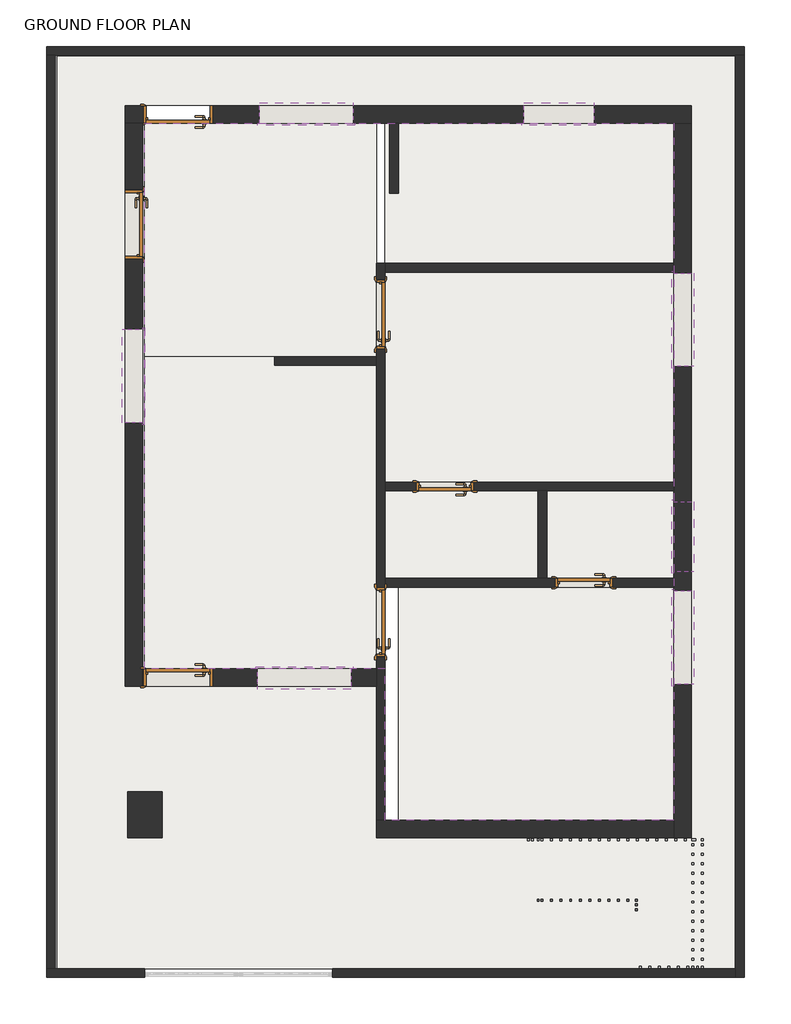
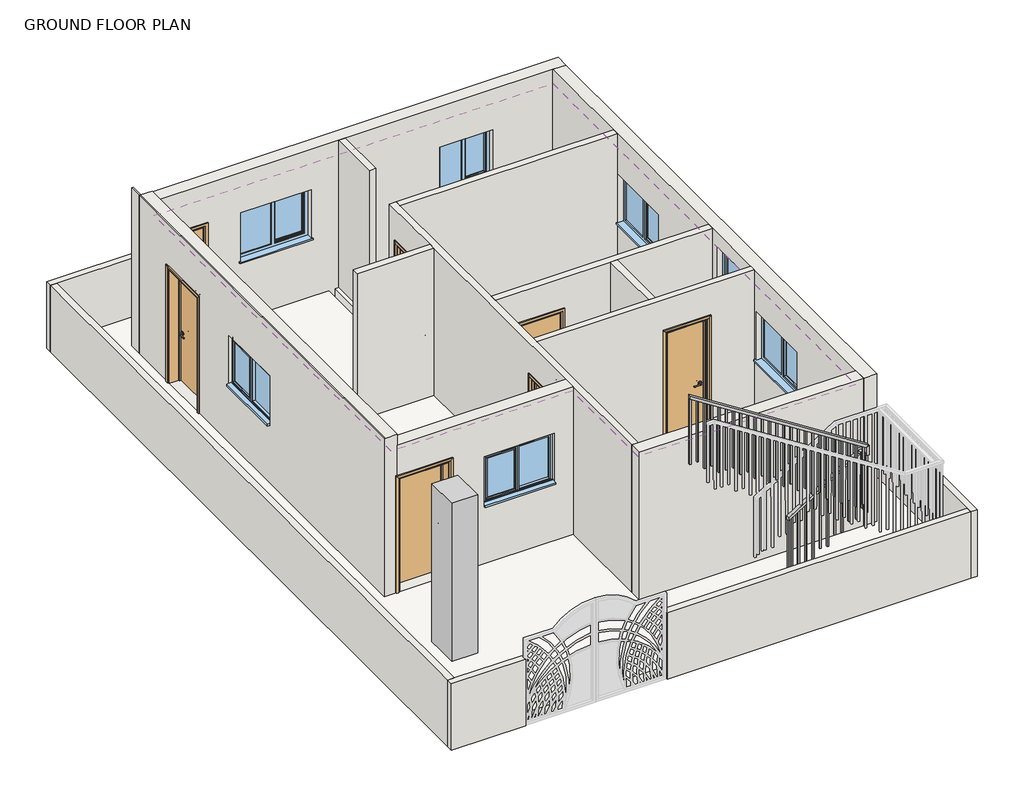
# One storey, part 1 of 23: 17 walls, 8 slabs, 7 doors, 7 windows, 1 column, 1 covering, 1 railing.
# Revit data of these elements (continued)
# Type "Windows_Sgl_Plain : V" (continued)
#   Rough Width = 3.0 ft
#   Rough Height = 2.985564 ft
#   Height = 2.985564 ft
#   Width = 3.0 ft
#   Heat Transfer Coefficient (U) = 5.5617 W/(m²·K)
#   Glazing Thickness = 0.07874 ft
#   FrameOffset - External = 0.164042 ft
#   Frame Depth = 0.213255 ft
#   Default Head Height = 6.922572 ft
#   Cill Depth = 0.287073 ft
#   Cavity Closer Width = 0.164042 ft
#   Cavity Closer Offset from Ext = 0.336286 ft
#   Cavity Closer Depth = 0.278871 ft
#   Vis - Cavity Closers = yes
#   Define Thermal Properties by = 1
#   Material Trim = Window Frame
#   Material Glass = Glass
#   Material Frame = Window Frame
#   Wall Closure = (empty or 0)
# Element 1 (IfcColumn, "Columns_Rectangular : 450x600mm")
#   Phase Created = New Construction
# Element 2 (IfcCovering)
#   Height Offset From Level = 8.5 ft
#   Phase Created = New Construction
#   Materials on its faces: "Gypsum Wall Board", "Metal Stud Layer"
# Elements 3, 4, 5, 6, 7 (IfcDoor, "Doors_IntSgl : D1")
#   Phase Created = New Construction
#   Materials on its faces: "Door - Architrave", "Door - Handle", "Door - Frame/Mullion (1)", "Door - Panel"
# Elements 8, 9 (IfcDoor, "Doors_IntSgl : D2")
#   Phase Created = New Construction
#   Materials on its faces: "Door - Architrave", "Door - Handle", "Door - Frame/Mullion (1)", "Door - Panel"
# Element 10 (IfcRailing, "1100mm")
#   Phase Created = New Construction
# Elements 11, 12 (IfcSlab, "BATHROOM FLOORING")
#   Height Offset From Level = 0.492 ft
#   Phase Created = New Construction
#   Materials on its faces: "Structure, Timber Joist/Rafter Layer", "BATHROOM FLOOR"
# Elements 13, 14 (IfcSlab, "BED ROOM FLOORING")
#   Height Offset From Level = 0.492 ft
#   Phase Created = New Construction
#   Materials on its faces: "Structure, Timber Joist/Rafter Layer", "BEDROOM FLOOR"
# Element 15 (IfcSlab, "DINING FLOORING")
#   Height Offset From Level = 0.492 ft
#   Phase Created = New Construction
#   Materials on its faces: "Structure, Timber Joist/Rafter Layer", "KITCHEN FLOOR"
# Element 16 (IfcSlab, "HALL FLOORING")
#   Height Offset From Level = 0.492 ft
#   Phase Created = New Construction
#   Materials on its faces: "Structure, Timber Joist/Rafter Layer", "HALL FLOOR"
# Element 17 (IfcSlab, "KITCHEN FLOOR")
#   Height Offset From Level = 0.492 ft
#   Phase Created = New Construction
#   Materials on its faces: "Structure, Timber Joist/Rafter Layer", "KITCHEN FLOOR"
# Element 18 (IfcSlab, "OUTER FLOORING")
#   Height Offset From Level = 0.492 ft
#   Phase Created = New Construction
#   Materials on its faces: "Structure, Timber Joist/Rafter Layer", "Concrete Masonry Units _High Density"
# Elements 19, 20, 21, 22, 23 (IfcWall)
#   Top Offset = -6.0 ft
#   Base Offset = 0.0 ft
#   wall height = 4.0 ft
#   Phase Created = New Construction
#   Base Constraint = GROUND FLOOR PLAN
#   Top Constraint = TYPICAL FLOOR LEVEL AND FFL
#   Materials on its faces: "Brick, Common"
# Elements 24, 25, 26, 27, 28 (IfcWall, "EXT WALL")
#   Top Offset = 0.0 ft
#   Base Offset = 0.0 ft
#   wall height = 10.0 ft
#   Phase Created = New Construction
#   Base Constraint = GROUND FLOOR PLAN
#   Top Constraint = TYPICAL FLOOR LEVEL AND FFL
#   Materials on its faces: "Brick, Common"
# Elements 29, 30, 31, 33, 34, 35 (IfcWall, "INT WALL")
#   Top Offset = 0.0 ft
#   Base Offset = 0.0 ft
#   wall height = 10.0 ft
#   Phase Created = New Construction
#   Base Constraint = GROUND FLOOR PLAN
#   Top Constraint = TYPICAL FLOOR LEVEL AND FFL
#   Materials on its faces: "Brick, Common"
# Element 32 (IfcWall, "INT WALL")
#   built-in parameter 1001111 = 0.010937 ft
#   Top Offset = 0.0 ft
#   Base Offset = 0.010937 ft
#   wall height = 9.989063 ft
#   Phase Created = New Construction
#   Base Constraint = GROUND FLOOR PLAN
#   Top Constraint = TYPICAL FLOOR LEVEL AND FFL
#   Materials on its faces: "Brick, Common"
# Elements 36, 37, 38, 39, 40 (IfcWindow, "Windows_Dbl_Plain : W1")
#   Mark = "W1"
#   Phase Created = New Construction
#   Materials on its faces: "Window Frame", "Glass"
# Element 41 (IfcWindow, "Windows_Dbl_Plain : W2")
#   Mark = "W2"
#   Phase Created = New Construction
#   Materials on its faces: "Window Frame", "Glass"
# Element 42 (IfcWindow, "Windows_Sgl_Plain : V")
#   Mark = "V"
#   Phase Created = New Construction
#   Materials on its faces: "Window Frame", "Glass"
# Materials
#   "Metal Stud Layer": class "Metal", colour RGB 127 127 127, transparency 0, Description = "Light gauge steel framing, thermal air layer", Cost = 0
#   "Gypsum Wall Board": class "Generic", colour RGB 249 249 249, transparency 0, Description = "Gypsum Wall Board", Cost = 0
#   "Door - Handle": colour RGB 0 0 0, transparency 0, Keynote = "P21", Cost = 0
#   "Door - Frame/Mullion (1)": class "Wood", colour RGB 212 179 113, transparency 0, Keynote = "L20", Cost = 0
#   "Door - Panel": class "Wood", colour RGB 210 159 95, transparency 0, Keynote = "L20", Cost = 0
#   "Door - Architrave": class "Wood", colour RGB 154 90 5, transparency 0, Keynote = "P20", Cost = 0
#   "BATHROOM FLOOR": class "Generic", colour RGB 120 120 120, transparency 0, Cost = 0
#   "Structure, Timber Joist/Rafter Layer": class "Wood", colour RGB 127 127 127, transparency 0, Description = "Timber framing, thermal airspace", Cost = 0
#   "BEDROOM FLOOR": class "Generic", colour RGB 120 120 120, transparency 0, Cost = 0
#   "KITCHEN FLOOR": class "Generic", colour RGB 120 120 120, transparency 0, Cost = 0
#   "HALL FLOOR": class "Generic", colour RGB 120 120 120, transparency 0, Cost = 0
#   "Concrete Masonry Units _High Density": class "Masonry", colour RGB 181 181 181, transparency 0, Description = "Concrete masonry units", Cost = 0
#   "Brick, Common": class "Masonry", colour RGB 170 100 105, transparency 0, Description = "Common brick", Cost = 0
#   "Window Frame": colour RGB 249 249 249, transparency 0, Keynote = "L10", Cost = 0
#   "Glass": class "Glass", colour RGB 0 128 192, transparency 0.9, Description = "Soda Lime Glass", Cost = 0
